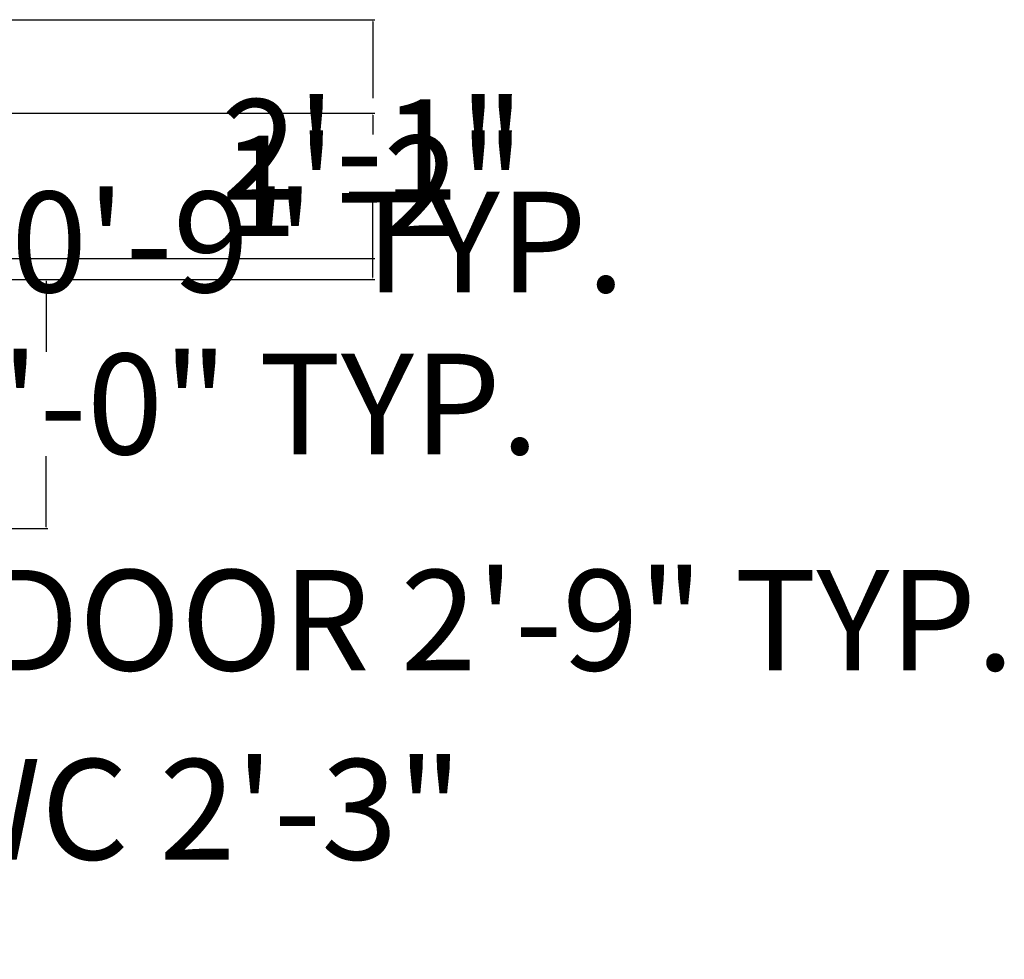
# Model space of a CAD drawing. Units: inches. Extents: x 2103 to 2702, y 2405 to 3142.
# Tile 7 of 7: x 2607 to 2702, y 2978 to 3069. Entities that reach past the tile are written whole.
import ezdxf

# ---------------------------------------------------------------- set-up
doc = ezdxf.new("R2010")
doc.units = ezdxf.units.IN
doc.layers.add('A-ANNO-DIMS', color=2, linetype='Continuous', lineweight=18)
doc.styles.get("Standard").update_dxf_attribs({"font": 'arial.ttf'})
doc.dimstyles.get("Standard").update_dxf_attribs({"dimtxt": 9.68, "dimasz": 0.18, "dimexe": 0.18, "dimexo": 0.0625, "dimgap": 0.09, "dimtad": 0, "dimtih": 1, "dimtoh": 1, "dimdec": 1, "dimzin": 0, "dimdsep": 46, "dimlunit": 3, "dimtxsty": 'Standard', "dimcen": 0.09, "dimadec": 0, "dimazin": 0, "dimtfac": 1, "dimtdec": 1, "dimtofl": 0, "dimtmove": 0, "dimatfit": 3, "dimfxl": 1, "dimtolj": 1, "dimtzin": 0, "dimarcsym": 0})

# ---------------------------------------------------------------- blocks, each defined once
blk = doc.blocks.new('*D20')
at = {"layer": 'A-ANNO-DIMS', "color": 0, "lineweight": -2, "transparency": 16777216}
for p, q in [((2606.493, 3043.846), (2610.21, 3043.846)), ((2610.03, 3043.666), (2610.03, 3036.878)), ((2610.03, 3020.026), (2610.03, 3026.813)), ((2606.493, 3019.846), (2610.21, 3019.846))]:
    blk.add_line(p, q, dxfattribs=at)
at = {"layer": 'A-ANNO-DIMS', "color": 0, "transparency": 16777216}
for points in [[(2610, 3043.666), (2610.06, 3043.666), (2610.03, 3043.846)], [(2610, 3020.026), (2610.06, 3020.026), (2610.03, 3019.846)]]:
    blk.add_solid(points, dxfattribs=at)
at = {"layer": 'Defpoints', "color": 0, "transparency": 16777216}
for p in [(2606.43, 3043.846), (2606.43, 3019.846), (2610.03, 3019.846)]:
    blk.add_point(p, dxfattribs=at)
at = {"layer": 'A-ANNO-DIMS', "color": 0, "transparency": 16777216, "insert": (2610.03, 3031.846), "char_height": 9.68, "attachment_point": 5}
blk.add_mtext('\\A1;VENT 2\'-0" TYP.', dxfattribs=at)
blk = doc.blocks.new('*D21')
at = {"layer": 'A-ANNO-DIMS', "color": 0, "lineweight": -2, "transparency": 16777216}
for p, q in [((2597.43, 3043.908), (2597.43, 3047.626)), ((2597.61, 3047.446), (2606.25, 3047.446)), ((2606.43, 3043.908), (2606.43, 3047.626)), ((2606.43, 3047.446), (2606.61, 3047.446))]:
    blk.add_line(p, q, dxfattribs=at)
at = {"layer": 'A-ANNO-DIMS', "color": 0, "transparency": 16777216}
for points in [[(2597.61, 3047.476), (2597.61, 3047.416), (2597.43, 3047.446)], [(2606.25, 3047.476), (2606.25, 3047.416), (2606.43, 3047.446)]]:
    blk.add_solid(points, dxfattribs=at)
at = {"layer": 'Defpoints', "color": 0, "transparency": 16777216}
for p in [(2606.43, 3047.446), (2597.43, 3043.846), (2606.43, 3043.846)]:
    blk.add_point(p, dxfattribs=at)
at = {"layer": 'A-ANNO-DIMS', "color": 0, "transparency": 16777216, "insert": (2636.202, 3047.446), "char_height": 9.68, "attachment_point": 5}
blk.add_mtext('\\A1;0\'-9" TYP.', dxfattribs=at)
blk = doc.blocks.new('*D24')
at = {"layer": 'A-ANNO-DIMS', "color": 0, "lineweight": -2, "transparency": 16777216}
for p, q in [((2530.307, 3015.94), (2530.307, 3010.852)), ((2563.445, 3015.94), (2563.445, 3010.852)), ((2530.487, 3011.032), (2563.265, 3011.032)), ((2563.445, 3011.032), (2563.625, 3011.032))]:
    blk.add_line(p, q, dxfattribs=at)
at = {"layer": 'A-ANNO-DIMS', "color": 0, "transparency": 16777216}
for points in [[(2530.487, 3011.062), (2530.487, 3011.002), (2530.307, 3011.032)], [(2563.265, 3011.062), (2563.265, 3011.002), (2563.445, 3011.032)]]:
    blk.add_solid(points, dxfattribs=at)
at = {"layer": 'Defpoints', "color": 0, "transparency": 16777216}
for p in [(2530.307, 3016.003), (2563.445, 3016.003), (2563.445, 3011.032)]:
    blk.add_point(p, dxfattribs=at)
at = {"layer": 'A-ANNO-DIMS', "color": 0, "transparency": 16777216, "insert": (2635.077, 3011.032), "char_height": 9.68, "attachment_point": 5}
blk.add_mtext('\\A1;BATH DOOR 2\'-9" TYP.', dxfattribs=at)
blk = doc.blocks.new('*D36')
at = {"layer": 'A-ANNO-DIMS', "color": 0, "lineweight": -2, "transparency": 16777216}
for p, q in [((2570.388, 2988.808), (2570.388, 2993.001)), ((2570.568, 2992.821), (2597.377, 2992.821)), ((2597.557, 2988.808), (2597.557, 2993.001)), ((2597.557, 2992.821), (2597.737, 2992.821))]:
    blk.add_line(p, q, dxfattribs=at)
at = {"layer": 'A-ANNO-DIMS', "color": 0, "transparency": 16777216}
for points in [[(2570.568, 2992.851), (2570.568, 2992.791), (2570.388, 2992.821)], [(2597.377, 2992.851), (2597.377, 2992.791), (2597.557, 2992.821)]]:
    blk.add_solid(points, dxfattribs=at)
at = {"layer": 'Defpoints', "color": 0, "transparency": 16777216}
for p in [(2597.557, 2992.821), (2570.388, 2988.745), (2597.557, 2988.745)]:
    blk.add_point(p, dxfattribs=at)
at = {"layer": 'A-ANNO-DIMS', "color": 0, "transparency": 16777216, "insert": (2624.034, 2992.821), "char_height": 9.68, "attachment_point": 5}
blk.add_mtext('\\A1;WC 2\'-3"', dxfattribs=at)
blk = doc.blocks.new('*D58')
at = {"layer": 'A-ANNO-DIMS', "color": 0, "lineweight": -2, "transparency": 16777216}
for p, q in [((2606.493, 3068.846), (2641.66, 3068.846)), ((2641.48, 3068.666), (2641.48, 3061.295)), ((2641.48, 3044.026), (2641.48, 3051.396)), ((2606.493, 3043.846), (2641.66, 3043.846))]:
    blk.add_line(p, q, dxfattribs=at)
at = {"layer": 'A-ANNO-DIMS', "color": 0, "transparency": 16777216}
for points in [[(2641.45, 3068.666), (2641.51, 3068.666), (2641.48, 3068.846)], [(2641.45, 3044.026), (2641.51, 3044.026), (2641.48, 3043.846)]]:
    blk.add_solid(points, dxfattribs=at)
at = {"layer": 'Defpoints', "color": 0, "transparency": 16777216}
for p in [(2606.43, 3068.846), (2606.43, 3043.846), (2641.48, 3043.846)]:
    blk.add_point(p, dxfattribs=at)
at = {"layer": 'A-ANNO-DIMS', "color": 0, "transparency": 16777216, "insert": (2641.48, 3056.346), "char_height": 9.68, "attachment_point": 5}
blk.add_mtext('\\A1;2\'-1"', dxfattribs=at)
blk = doc.blocks.new('*D69')
at = {"layer": 'A-ANNO-DIMS', "color": 0, "lineweight": -2, "transparency": 16777216}
for p, q in [((2537.493, 3059.846), (2641.66, 3059.846)), ((2641.48, 3059.666), (2641.48, 3057.795)), ((2641.48, 3046.026), (2641.48, 3047.896)), ((2537.493, 3045.846), (2641.66, 3045.846))]:
    blk.add_line(p, q, dxfattribs=at)
at = {"layer": 'A-ANNO-DIMS', "color": 0, "transparency": 16777216}
for points in [[(2641.45, 3059.666), (2641.51, 3059.666), (2641.48, 3059.846)], [(2641.45, 3046.026), (2641.51, 3046.026), (2641.48, 3045.846)]]:
    blk.add_solid(points, dxfattribs=at)
at = {"layer": 'Defpoints', "color": 0, "transparency": 16777216}
for p in [(2537.43, 3059.846), (2641.48, 3059.846), (2537.43, 3045.846)]:
    blk.add_point(p, dxfattribs=at)
at = {"layer": 'A-ANNO-DIMS', "color": 0, "transparency": 16777216, "insert": (2641.48, 3052.846), "char_height": 9.68, "attachment_point": 5}
blk.add_mtext('\\A1;1\'-2"', dxfattribs=at)

msp = doc.modelspace()

# ---------------------------------------------------------------- dimensions: what is measured, and where the dimension line sits
at = {"layer": 'A-ANNO-DIMS'}
for base, p1, p2, picture, middle in [((2641.48, 3043.846), (2606.43, 3068.846), (2606.43, 3043.846), '*D58', (2641.48, 3056.346)), ((2641.48, 3059.846), (2537.43, 3045.846), (2537.43, 3059.846), '*D69', (2641.48, 3052.846))]:
    dim = msp.add_linear_dim(base=base, p1=p1, p2=p2, angle=90, dimstyle='Standard', override={"dimdec": 1, "dimlfac": 1, "dimrnd": 0, "dimzin": 1, "dimdsep": 46, "dimlunit": 4, "dimfrac": 2}, dxfattribs=at)
    dim.commit()
    dim.dimension.update_dxf_attribs({"geometry": picture, "text_midpoint": middle})
for base, p1, p2, text, picture, middle in [((2606.43, 3047.446), (2597.43, 3043.846), (2606.43, 3043.846), '<> TYP.', '*D21', (2636.202, 3047.446)), ((2563.445, 3011.032), (2530.307, 3016.003), (2563.445, 3016.003), 'BATH DOOR <> TYP.', '*D24', (2635.077, 3011.032)), ((2597.557, 2992.821), (2570.388, 2988.745), (2597.557, 2988.745), 'WC <>', '*D36', (2624.034, 2992.821))]:
    dim = msp.add_linear_dim(base=base, p1=p1, p2=p2, text=text, dimstyle='Standard', override={"dimdec": 1, "dimlfac": 1, "dimrnd": 0, "dimzin": 1, "dimdsep": 46, "dimlunit": 4, "dimfrac": 2}, dxfattribs=at)
    dim.commit()
    dim.dimension.update_dxf_attribs({"geometry": picture, "text_midpoint": middle})
dim = msp.add_linear_dim(base=(2610.03, 3019.846), p1=(2606.43, 3043.846), p2=(2606.43, 3019.846), angle=270, text='VENT <> TYP.', dimstyle='Standard', override={"dimdec": 1, "dimlfac": 1, "dimrnd": 0, "dimzin": 1, "dimdsep": 46, "dimlunit": 4, "dimfrac": 2}, dxfattribs=at)
dim.commit()
dim.dimension.update_dxf_attribs({"geometry": '*D20', "text_midpoint": (2610.03, 3031.846)})

doc.saveas('drawing.dxf')
